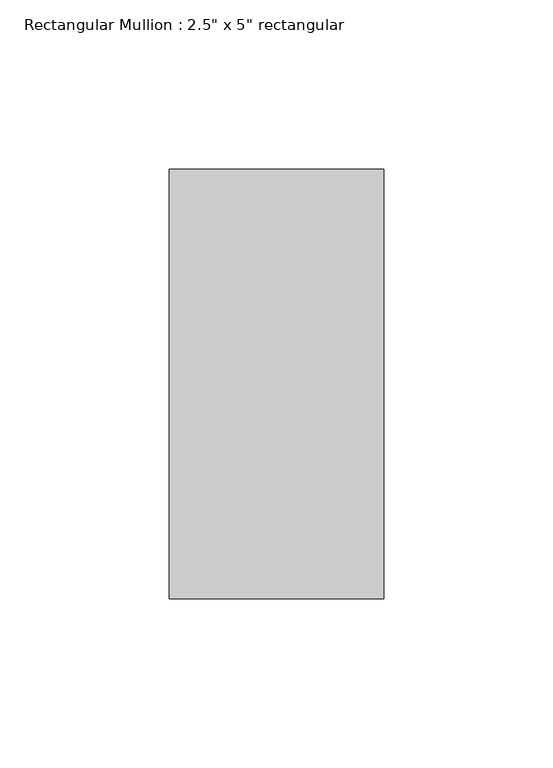
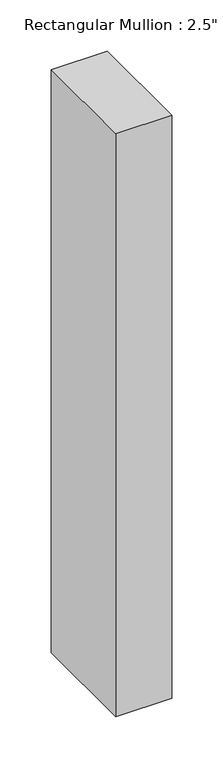
"""IFC4 building model written with IfcOpenShell, lengths in millimetres: member geometry."""

from ifc_helpers import new_model, si_unit, frame, origin, place, context, project, spatial, polyline, outline, extrude, source, transform, mapped, element, save


def member_c0b2eca9(model_context):
    return source(origin(), model_context, "Body", "SweptSolid", [
        extrude(outline(polyline([(0.0, 63.5), (0.0, -63.5), (-63.5, -63.5), (-63.5, 63.5), (0.0, 63.5)])), frame((0.0, 0.0, -697.4776209), z_axis=(0.0, 0.0, 1.0), x_axis=(1.0, 0.0, 0.0)), (0.0, 0.0, 1.0), 697.4776209),
    ])


if __name__ == "__main__":
    model = new_model("IFC4")
    model_context = context("Model", 3, world=origin())
    ifc_project = project(units=[si_unit("LENGTHUNIT", "METRE", prefix="MILLI")], contexts=[model_context])
    site = spatial("IfcSite", under=ifc_project)
    building = spatial("IfcBuilding", under=site)
    placement = place(None, origin())
    member_shape = member_c0b2eca9(model_context)
    element("IfcMember", 1, ObjectType="Rectangular Mullion : 2.5\" x 5\" rectangular", at=placement, inside=building, context=model_context, shape_type="MappedRepresentation", body=[
        mapped(member_shape, transform((0.0, 0.0, 0.0), x_axis=(1.0, 0.0, 0.0), y_axis=(0.0, 1.0, 0.0), z_axis=(0.0, 0.0, 1.0))),
    ])
    save(model, "model.ifc")

# Revit data of these elements
# Type "Rectangular Mullion : 2.5\" x 5\" rectangular"
#   built-in parameter 1007304 = 0.416667 (stored number, unit not read)
#   built-in parameter 1007301 = 0.104167 (stored number, unit not read)
#   built-in parameter 1007300 = 0.104167 (stored number, unit not read)
# Element 1 (IfcMember, "Rectangular Mullion : 2.5\" x 5\" rectangular")
#   Materials on its faces: "Aluminum"
# Materials
#   "Aluminum": class "Metal", colour RGB 247 247 247, transparency 0, Description = "Aluminum 6061", Cost = 0
